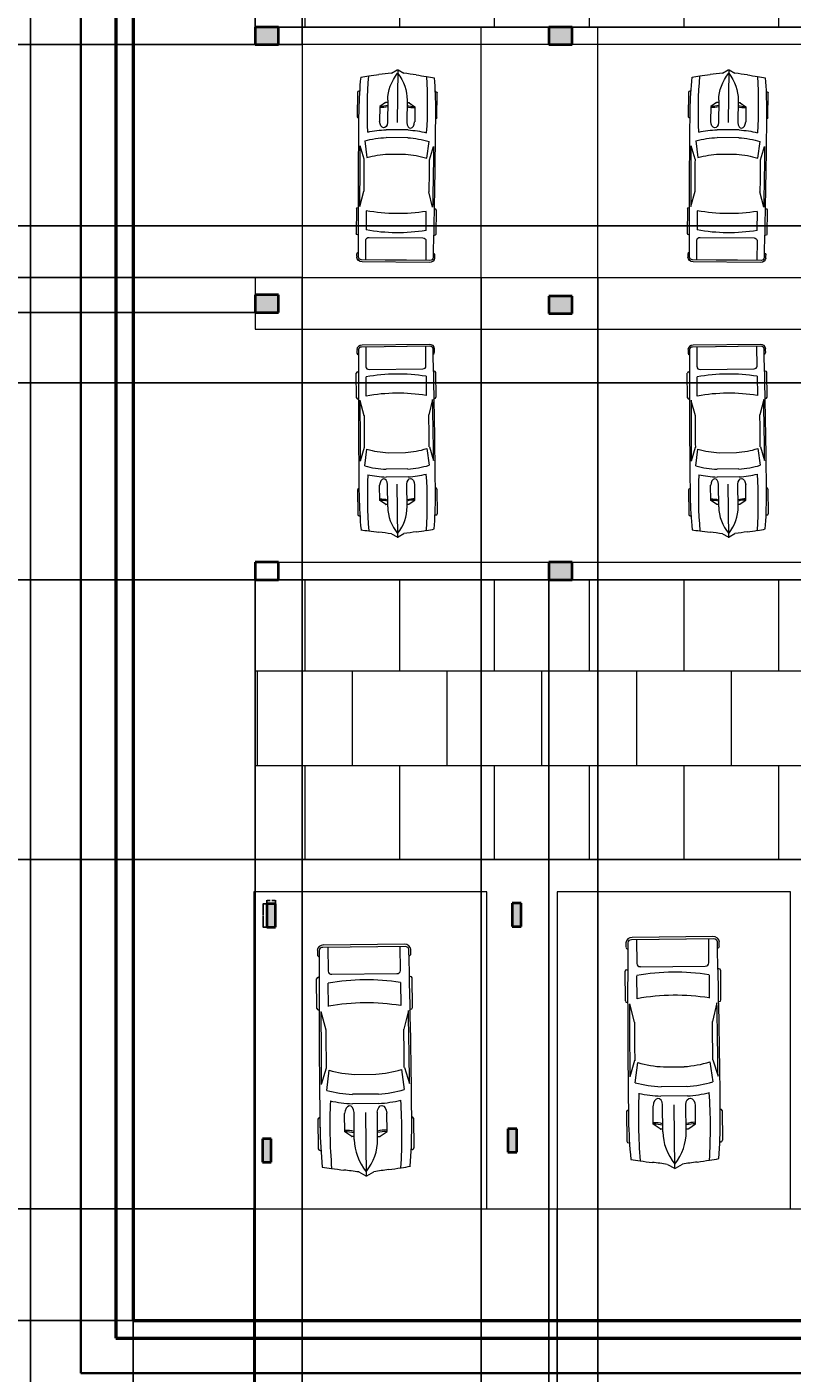
# Model space of a CAD drawing. Units: inches. Extents: x 154617 to 156384, y 250671 to 252576.
# Tile 3 of 6: x 155207 to 155601, y 251035 to 251728. Entities that reach past the tile are written whole.
import ezdxf

# ---------------------------------------------------------------- set-up
doc = ezdxf.new("R2010")
doc.units = ezdxf.units.IN
for name, color, linetype, lineweight in [('A-ANNO-DIMS', 2, 'Continuous', 18), ('A-EQPM-VEHI', 9, 'Continuous', 13), ('A-FLOR-DRIV', 5, 'Continuous', 25), ('A-FLOR-PATT', 112, 'Continuous', 13), ('A-FLOR-PRKG', 4, 'Continuous', 18), ('C-PROP', 5, 'Continuous', 35), ('C-ROAD', 7, 'Continuous', 25), ('pillars', 6, 'Continuous', 40), ('walls', 4, 'Continuous', 50)]:
    doc.layers.add(name, color=color, linetype=linetype, lineweight=lineweight)
doc.styles.get("Standard").update_dxf_attribs({"font": 'arial.ttf'})
doc.dimstyles.get("Standard").update_dxf_attribs({"dimtxt": 0.18, "dimasz": 0.18, "dimexe": 0.18, "dimexo": 0.0625, "dimgap": 0.09, "dimtad": 0, "dimtih": 1, "dimtoh": 1, "dimdec": 4, "dimzin": 0, "dimdsep": 46, "dimtxsty": 'Standard', "dimcen": 0.09, "dimadec": 0, "dimazin": 0, "dimtfac": 1, "dimtdec": 4, "dimtofl": 0, "dimtmove": 0, "dimatfit": 3, "dimfxl": 1, "dimtolj": 1, "dimtzin": 0, "dimarcsym": 0})

# ---------------------------------------------------------------- blocks, each defined once
blk = doc.blocks.new('*U2')
for p, q in [((21.1, 37.4), (21.1, 36.8)), ((46.6, 38.9), (22.4, 38.9)), ((47.8, 37.4), (47.8, 37.4)), ((88, 31.9), (74.8, 35.9)), ((134.3, 35.6), (119.3, 31.8)), ((135.5, 37.1), (135.5, 37.4)), ((136.7, 38.9), (160.9, 38.9)), ((162.1, 37.4), (162.1, 36.8)), ((186.5, -33.5), (186.5, 33.5)), ((70, 31.5), (86.4, 29.4)), ((138.4, 29.4), (157.2, 29.4)), ((164.5, 26.4), (164.5, -26.4)), ((186.5, 29.4), (167, 29.4)), ((188.4, -32.8), (188.4, 32.8)), ((32.1, 9.5), (32.1, 11.2)), ((32.3, 11.6), (36.1, 17.2)), ((36.1, 17.2), (50.9, 17.2)), ((3.3, 6.1), (0.1, 0.4)), ((29.8, 9.5), (51.7, 9.5)), ((58.9, -10.8), (58.9, 10.8)), ((66.6, -10.5), (66.6, 10.5)), ((82.7, 8.5), (82.7, -8.5)), ((186.5, -10.5), (186.5, 10.5)), ((0, 0), (51.7, 0)), ((0.1, -0.4), (3.3, -6.1)), ((29.8, -9.5), (51.7, -9.5)), ((32.1, -9.5), (32.1, -11.2)), ((32.3, -11.6), (36.1, -17.2)), ((36.1, -17.2), (50.9, -17.2)), ((86.4, -29.4), (70, -31.5)), ((88, -31.9), (74.8, -35.9)), ((134.3, -35.6), (119.3, -31.8)), ((157.2, -29.4), (138.4, -29.4)), ((167, -29.4), (186.5, -29.4)), ((21.1, -37.4), (21.1, -36.8)), ((46.6, -38.9), (22.4, -38.9)), ((47.8, -37.4), (47.8, -37.4)), ((135.5, -37.1), (135.5, -37.4)), ((136.7, -38.9), (160.9, -38.9)), ((162.1, -37.4), (162.1, -36.8))]:
    blk.add_line(p, q)
for centre, major_axis, ratio, start_param, end_param in [((266, -27.5), (0, 313.3), 0.842304, 1.367076, 1.39176), ((41.2, -490.9), (0, 528.2), 0.842304, 0.00281, 0.075598), ((22.4, 37.4), (0, -1.48), 0.842304, 3.141593, 4.712389), ((64.5, -10555.6), (0, 10593), 0.842304, -0.013397, 0.002797), ((46.6, 37.4), (0, 1.48), 0.842304, -1.570796, 0), ((64.5, -10555.6), (0, -10591.5), 0.842304, 3.133765, 3.140441), ((136.7, 37.4), (0, -1.48), 0.842304, 3.141593, 4.712389), ((160.9, 37.4), (0, 1.48), 0.842304, -1.570796, 0), ((180.6, 35.8), (0, 2.22), 0.842304, -0.013017, 1.249894), ((64.5, -10556.4), (0, 10595.3), 0.842304, -0.013397, -0.013017), ((184, 32.8), (0, -5.25), 0.842304, 1.570796, 3.128196), ((184, 33.5), (0, -2.96), 0.842304, 1.570796, 3.128196), ((259.2, -27.5), (0, -305.3), 0.842304, 4.528606, 4.561838), ((37.5, -594), (0, -623.3), 0.842304, 3.096046, 3.200911), ((134.4, 5.4), (0, -89.8), 0.842304, 4.449482, 4.652344), ((135.3, 5.4), (0, 81.8), 0.842304, 1.245306, 1.50788), ((149.6, 2.8), (0, -79.6), 0.842304, 4.372215, 4.640744), ((95.8, -3666.4), (0, -3698.2), 0.842304, 3.134049, 3.144098), ((17.1, 0), (0, 147), 0.842304, 4.511394, 4.913384), ((35.9, 0), (0, 147), 0.842304, 4.511394, 4.913384), ((167, 26.4), (0, 2.96), 0.842304, 0, 1.570796), ((-204.5, 52.4), (0, -251), 0.842304, 1.385369, 1.434372), ((32.7, 11.2), (0, 0.74), 0.842304, 0.879714, 1.570796), ((13, 17), (0, 27.4), 0.842304, 4.435146, 4.718221), ((14.2, 17), (0, 27.4), 0.842304, 4.435146, 4.718221), ((50.8, 13.3), (6.34, -0.36), 0.603834, -1.395552, 1.581315), ((0.6, 0), (0, -0.74), 0.842304, 4.131459, 5.293319), ((29.8, -46.7), (0, 56.2), 0.842304, 0, 0.590319), ((-204.5, -52.4), (0, 251), 0.842304, -1.434372, -1.385369), ((29.8, 46.7), (0, 56.2), 0.842304, 2.551274, 3.141593), ((13, -17), (0, -27.4), 0.842304, 1.564964, 1.848039), ((14.2, -17), (0, -27.4), 0.842304, 1.564964, 1.848039), ((134.4, -5.4), (0, -89.8), 0.842304, -1.510751, -1.307889), ((135.3, -5.4), (0, -81.8), 0.842304, -1.50788, -1.245306), ((149.6, -2.8), (0, -79.6), 0.842304, -1.499151, -1.230623), ((259.2, 27.5), (0, 305.3), 0.842304, 1.721348, 1.754579), ((32.7, -11.2), (0, -0.74), 0.842304, 4.712389, 5.403472), ((266, 27.5), (0, 313.3), 0.842304, 1.749832, 1.774517), ((37.5, 594), (0, -623.3), 0.842304, -0.059319, 0.045547), ((95.8, 3666.4), (0, -3698.2), 0.842304, -0.002505, 0.007544), ((167, -26.4), (0, -2.96), 0.842304, 4.712389, 6.283185), ((184, -32.8), (0, -5.25), 0.842304, 0.013397, 1.570796), ((41.2, 490.9), (0, -528.2), 0.842304, -0.075598, -0.00281), ((22.4, -37.4), (0, 1.48), 0.842304, 1.570796, 3.141593), ((64.5, 10555.6), (0, 10593), 0.842304, 3.138796, 3.15499), ((46.6, -37.4), (0, -1.48), 0.842304, 0, 1.570796), ((64.5, 10555.6), (0, -10591.5), 0.842304, 0.001152, 0.007828), ((136.7, -37.4), (0, -1.48), 0.842304, -1.570796, 0), ((160.9, -37.4), (0, 1.48), 0.842304, 3.141593, 4.712389), ((180.6, -35.8), (0, -2.22), 0.842304, -1.249894, 0.013017), ((64.5, 10556.4), (0, 10595.3), 0.842304, 3.15461, 3.15499), ((184, -33.5), (0, 2.96), 0.842304, 3.15499, 4.712389)]:
    blk.add_ellipse(centre, major_axis=major_axis, ratio=ratio, start_param=start_param, end_param=end_param)
at = {"extrusion": (0, 0, -1)}
blk.add_ellipse((50.8, -13.3), major_axis=(6.34, 0.36), ratio=0.603834, start_param=-1.395552, end_param=1.581315, dxfattribs=at)
blk = doc.blocks.new('COL-RECT-12x9')
h = blk.add_hatch(color=256)
h.dxf.hatch_style = 1
h.paths.add_polyline_path([(12.01, 0), (12.01, 9), (0, 9), (0, 0)])
for p, q in [((12.01, 9), (0, 9)), ((0, 9), (0, 0)), ((12.01, 0), (12.01, 9)), ((0, 0), (12.01, 0))]:
    blk.add_line(p, q)
blk = doc.blocks.new('COL-NARROW-4_5x12')
h = blk.add_hatch(color=256)
h.dxf.hatch_style = 1
h.paths.add_polyline_path([(4.5, 12.01), (0, 12.01), (0, 0), (4.5, 0)])
for p, q in [((4.5, 12.01), (0, 12.01)), ((0, 12.01), (0, 0)), ((4.5, 0), (4.5, 12.01)), ((0, 0), (4.5, 0))]:
    blk.add_line(p, q)
blk = doc.blocks.new('PARKING-BAY-U')
for p, q in [((120, 163.22), (0, 163.22)), ((0, 163.22), (0, 0)), ((120, 0), (120, 163.22))]:
    blk.add_line(p, q)
blk = doc.blocks.new('*D13')
at = {"layer": 'A-ANNO-DIMS', "color": 0, "lineweight": -2, "transparency": 16777216}
for p, q in [((155330.71, 251276.59), (155328.79, 251276.59)), ((155328.97, 251276.41), (155328.97, 251270.76)), ((155330.71, 251264.57), (155328.79, 251264.57)), ((155328.97, 251264.75), (155328.97, 251270.4))]:
    blk.add_line(p, q, dxfattribs=at)
at = {"layer": 'A-ANNO-DIMS', "color": 0, "transparency": 16777216}
for points in [[(155328.94, 251276.41), (155329, 251276.41), (155328.97, 251276.59)], [(155328.94, 251264.75), (155329, 251264.75), (155328.97, 251264.57)]]:
    blk.add_solid(points, dxfattribs=at)
at = {"layer": 'Defpoints', "color": 0, "transparency": 16777216}
for p in [(155330.77, 251276.59), (155328.97, 251264.57), (155330.77, 251264.57)]:
    blk.add_point(p, dxfattribs=at)
at = {"layer": 'A-ANNO-DIMS', "color": 0, "transparency": 16777216, "insert": (155328.97, 251270.58), "char_height": 0.18, "attachment_point": 5}
blk.add_mtext('\\A1;COLUMN 12 TYP.', dxfattribs=at)
blk = doc.blocks.new('*D14')
at = {"layer": 'A-ANNO-DIMS', "color": 0, "lineweight": -2, "transparency": 16777216}
for p, q in [((155330.77, 251276.65), (155330.77, 251278.57)), ((155330.95, 251278.39), (155332.56, 251278.39)), ((155335.09, 251278.39), (155333.48, 251278.39)), ((155335.27, 251276.65), (155335.27, 251278.57))]:
    blk.add_line(p, q, dxfattribs=at)
at = {"layer": 'A-ANNO-DIMS', "color": 0, "transparency": 16777216}
for points in [[(155330.95, 251278.42), (155330.95, 251278.36), (155330.77, 251278.39)], [(155335.09, 251278.42), (155335.09, 251278.36), (155335.27, 251278.39)]]:
    blk.add_solid(points, dxfattribs=at)
at = {"layer": 'Defpoints', "color": 0, "transparency": 16777216}
for p in [(155330.77, 251278.39), (155330.77, 251276.59), (155335.27, 251276.59)]:
    blk.add_point(p, dxfattribs=at)
at = {"layer": 'A-ANNO-DIMS', "color": 0, "transparency": 16777216, "insert": (155333.02, 251278.39), "char_height": 0.18, "attachment_point": 5}
blk.add_mtext('\\A1;5 TYP.', dxfattribs=at)
blk = doc.blocks.new('*D30')
at = {"layer": 'A-ANNO-DIMS', "color": 0, "lineweight": -2, "transparency": 16777216}
for p, q in [((155324.78, 251581.16), (154616.73, 251581.16)), ((154616.91, 251580.98), (154616.91, 251512.53)), ((154616.91, 251443.71), (154616.91, 251512.16)), ((155324.78, 251443.53), (154616.73, 251443.53))]:
    blk.add_line(p, q, dxfattribs=at)
at = {"layer": 'A-ANNO-DIMS', "color": 0, "transparency": 16777216}
for points in [[(154616.88, 251580.98), (154616.94, 251580.98), (154616.91, 251581.16)], [(154616.88, 251443.71), (154616.94, 251443.71), (154616.91, 251443.53)]]:
    blk.add_solid(points, dxfattribs=at)
at = {"layer": 'Defpoints', "color": 0, "transparency": 16777216}
for p in [(154616.91, 251581.16), (155324.84, 251581.16), (155324.84, 251443.53)]:
    blk.add_point(p, dxfattribs=at)
at = {"layer": 'A-ANNO-DIMS', "color": 0, "transparency": 16777216, "insert": (154616.91, 251512.35), "char_height": 0.18, "attachment_point": 5}
blk.add_mtext('\\A1;137.64', dxfattribs=at)
blk = doc.blocks.new('*D31')
at = {"layer": 'A-ANNO-DIMS', "color": 0, "lineweight": -2, "transparency": 16777216}
for p, q in [((155324.78, 251719.03), (154616.73, 251719.03)), ((154616.91, 251718.85), (154616.91, 251650.28)), ((154616.91, 251581.34), (154616.91, 251649.91)), ((155324.78, 251581.16), (154616.73, 251581.16))]:
    blk.add_line(p, q, dxfattribs=at)
at = {"layer": 'A-ANNO-DIMS', "color": 0, "transparency": 16777216}
for points in [[(154616.88, 251718.85), (154616.94, 251718.85), (154616.91, 251719.03)], [(154616.88, 251581.34), (154616.94, 251581.34), (154616.91, 251581.16)]]:
    blk.add_solid(points, dxfattribs=at)
at = {"layer": 'Defpoints', "color": 0, "transparency": 16777216}
for p in [(154616.91, 251719.03), (155324.84, 251719.03), (155324.84, 251581.16)]:
    blk.add_point(p, dxfattribs=at)
at = {"layer": 'A-ANNO-DIMS', "color": 0, "transparency": 16777216, "insert": (154616.91, 251650.1), "char_height": 0.18, "attachment_point": 5}
blk.add_mtext('\\A1;137.86', dxfattribs=at)
blk = doc.blocks.new('*D32')
at = {"layer": 'A-ANNO-DIMS', "color": 0, "lineweight": -2, "transparency": 16777216}
for p, q in [((155324.78, 251873.03), (154616.73, 251873.03)), ((154616.91, 251872.85), (154616.91, 251796.21)), ((154616.91, 251719.21), (154616.91, 251795.84)), ((155324.78, 251719.03), (154616.73, 251719.03))]:
    blk.add_line(p, q, dxfattribs=at)
at = {"layer": 'A-ANNO-DIMS', "color": 0, "transparency": 16777216}
for points in [[(154616.88, 251872.85), (154616.94, 251872.85), (154616.91, 251873.03)], [(154616.88, 251719.21), (154616.94, 251719.21), (154616.91, 251719.03)]]:
    blk.add_solid(points, dxfattribs=at)
at = {"layer": 'Defpoints', "color": 0, "transparency": 16777216}
for p in [(154616.91, 251873.03), (155324.84, 251873.03), (155324.84, 251719.03)]:
    blk.add_point(p, dxfattribs=at)
at = {"layer": 'A-ANNO-DIMS', "color": 0, "transparency": 16777216, "insert": (154616.91, 251796.03), "char_height": 0.18, "attachment_point": 5}
blk.add_mtext('\\A1;154', dxfattribs=at)
blk = doc.blocks.new('*D33')
at = {"layer": 'A-ANNO-DIMS', "color": 0, "lineweight": -2, "transparency": 16777216}
for p, q in [((155324.78, 251443.53), (154616.73, 251443.53)), ((154616.91, 251443.35), (154616.91, 251371.71)), ((154616.91, 251299.71), (154616.91, 251371.35)), ((155324.78, 251299.53), (154616.73, 251299.53))]:
    blk.add_line(p, q, dxfattribs=at)
at = {"layer": 'A-ANNO-DIMS', "color": 0, "transparency": 16777216}
for points in [[(154616.88, 251443.35), (154616.94, 251443.35), (154616.91, 251443.53)], [(154616.88, 251299.71), (154616.94, 251299.71), (154616.91, 251299.53)]]:
    blk.add_solid(points, dxfattribs=at)
at = {"layer": 'Defpoints', "color": 0, "transparency": 16777216}
for p in [(154616.91, 251443.53), (155324.84, 251443.53), (155324.84, 251299.53)]:
    blk.add_point(p, dxfattribs=at)
at = {"layer": 'A-ANNO-DIMS', "color": 0, "transparency": 16777216, "insert": (154616.91, 251371.53), "char_height": 0.18, "attachment_point": 5}
blk.add_mtext('\\A1;144', dxfattribs=at)
blk = doc.blocks.new('*D34')
at = {"layer": 'A-ANNO-DIMS', "color": 0, "lineweight": -2, "transparency": 16777216}
for p, q in [((155324.78, 251299.53), (154616.73, 251299.53)), ((154616.91, 251299.35), (154616.91, 251209.71)), ((154616.91, 251119.71), (154616.91, 251209.34)), ((155324, 251119.53), (154616.73, 251119.53))]:
    blk.add_line(p, q, dxfattribs=at)
at = {"layer": 'A-ANNO-DIMS', "color": 0, "transparency": 16777216}
for points in [[(154616.88, 251299.35), (154616.94, 251299.35), (154616.91, 251299.53)], [(154616.88, 251119.71), (154616.94, 251119.71), (154616.91, 251119.53)]]:
    blk.add_solid(points, dxfattribs=at)
at = {"layer": 'Defpoints', "color": 0, "transparency": 16777216}
for p in [(154616.91, 251299.53), (155324.84, 251299.53), (155324.06, 251119.53)]:
    blk.add_point(p, dxfattribs=at)
at = {"layer": 'A-ANNO-DIMS', "color": 0, "transparency": 16777216, "insert": (154616.91, 251209.53), "char_height": 0.18, "attachment_point": 5}
blk.add_mtext('\\A1;180', dxfattribs=at)
blk = doc.blocks.new('*D35')
at = {"layer": 'A-ANNO-DIMS', "color": 0, "lineweight": -2, "transparency": 16777216}
for p, q in [((155262.03, 251119.53), (154616.73, 251119.53)), ((154616.91, 251119.35), (154616.91, 251090.96)), ((154616.91, 251062.21), (154616.91, 251090.59)), ((155262.03, 251062.03), (154616.73, 251062.03))]:
    blk.add_line(p, q, dxfattribs=at)
at = {"layer": 'A-ANNO-DIMS', "color": 0, "transparency": 16777216}
for points in [[(154616.88, 251119.35), (154616.94, 251119.35), (154616.91, 251119.53)], [(154616.88, 251062.21), (154616.94, 251062.21), (154616.91, 251062.03)]]:
    blk.add_solid(points, dxfattribs=at)
at = {"layer": 'Defpoints', "color": 0, "transparency": 16777216}
for p in [(154616.91, 251119.53), (155262.1, 251119.53), (155262.1, 251062.03)]:
    blk.add_point(p, dxfattribs=at)
at = {"layer": 'A-ANNO-DIMS', "color": 0, "transparency": 16777216, "insert": (154616.91, 251090.78), "char_height": 0.18, "attachment_point": 5}
blk.add_mtext('\\A1;57.5', dxfattribs=at)
blk = doc.blocks.new('*D36')
at = {"layer": 'A-ANNO-DIMS', "color": 0, "lineweight": -2, "transparency": 16777216}
for p, q in [((155324.84, 251443.46), (155324.84, 250671.2)), ((155475.98, 251443.46), (155475.98, 250671.2)), ((155325.02, 250671.38), (155399.96, 250671.38)), ((155475.8, 250671.38), (155400.87, 250671.38))]:
    blk.add_line(p, q, dxfattribs=at)
at = {"layer": 'A-ANNO-DIMS', "color": 0, "transparency": 16777216}
for points in [[(155325.02, 250671.41), (155325.02, 250671.35), (155324.84, 250671.38)], [(155475.8, 250671.41), (155475.8, 250671.35), (155475.98, 250671.38)]]:
    blk.add_solid(points, dxfattribs=at)
at = {"layer": 'Defpoints', "color": 0, "transparency": 16777216}
for p in [(155324.84, 251443.53), (155475.98, 251443.53), (155475.98, 250671.38)]:
    blk.add_point(p, dxfattribs=at)
at = {"layer": 'A-ANNO-DIMS', "color": 0, "transparency": 16777216, "insert": (155400.41, 250671.38), "char_height": 0.18, "attachment_point": 5}
blk.add_mtext('\\A1;151.14', dxfattribs=at)
blk = doc.blocks.new('*D37')
at = {"layer": 'A-ANNO-DIMS', "color": 0, "lineweight": -2, "transparency": 16777216}
for p, q in [((155475.98, 251443.46), (155475.98, 250671.2)), ((155654.61, 251443.46), (155654.61, 250671.2)), ((155476.16, 250671.38), (155564.84, 250671.38)), ((155654.43, 250671.38), (155565.75, 250671.38))]:
    blk.add_line(p, q, dxfattribs=at)
at = {"layer": 'A-ANNO-DIMS', "color": 0, "transparency": 16777216}
for points in [[(155476.16, 250671.41), (155476.16, 250671.35), (155475.98, 250671.38)], [(155654.43, 250671.41), (155654.43, 250671.35), (155654.61, 250671.38)]]:
    blk.add_solid(points, dxfattribs=at)
at = {"layer": 'Defpoints', "color": 0, "transparency": 16777216}
for p in [(155475.98, 251443.53), (155654.61, 251443.53), (155654.61, 250671.38)]:
    blk.add_point(p, dxfattribs=at)
at = {"layer": 'A-ANNO-DIMS', "color": 0, "transparency": 16777216, "insert": (155565.3, 250671.38), "char_height": 0.18, "attachment_point": 5}
blk.add_mtext('\\A1;178.63', dxfattribs=at)
blk = doc.blocks.new('*D40')
at = {"layer": 'A-ANNO-DIMS', "color": 0, "lineweight": -2, "transparency": 16777216}
for p, q in [((155262.1, 251119.46), (155262.1, 250671.2)), ((155324.06, 251119.46), (155324.06, 250671.2)), ((155262.28, 250671.38), (155292.69, 250671.38)), ((155323.88, 250671.38), (155293.47, 250671.38))]:
    blk.add_line(p, q, dxfattribs=at)
at = {"layer": 'A-ANNO-DIMS', "color": 0, "transparency": 16777216}
for points in [[(155262.28, 250671.41), (155262.28, 250671.35), (155262.1, 250671.38)], [(155323.88, 250671.41), (155323.88, 250671.35), (155324.06, 250671.38)]]:
    blk.add_solid(points, dxfattribs=at)
at = {"layer": 'Defpoints', "color": 0, "transparency": 16777216}
for p in [(155262.1, 251119.53), (155324.06, 251119.53), (155324.06, 250671.38)]:
    blk.add_point(p, dxfattribs=at)
at = {"layer": 'A-ANNO-DIMS', "color": 0, "transparency": 16777216, "insert": (155293.08, 250671.38), "char_height": 0.18, "attachment_point": 5}
blk.add_mtext('\\A1;61.97', dxfattribs=at)
blk = doc.blocks.new('*D55')
at = {"layer": 'A-ANNO-DIMS', "color": 0, "lineweight": -2, "transparency": 16777216}
for p, q in [((155844.53, 251625.8), (154616.73, 251625.8)), ((154616.91, 251625.62), (154616.91, 251585.48)), ((154616.91, 251544.98), (154616.91, 251585.12)), ((155844.53, 251544.8), (154616.73, 251544.8))]:
    blk.add_line(p, q, dxfattribs=at)
at = {"layer": 'A-ANNO-DIMS', "color": 0, "transparency": 16777216}
for points in [[(154616.88, 251625.62), (154616.94, 251625.62), (154616.91, 251625.8)], [(154616.88, 251544.98), (154616.94, 251544.98), (154616.91, 251544.8)]]:
    blk.add_solid(points, dxfattribs=at)
at = {"layer": 'Defpoints', "color": 0, "transparency": 16777216}
for p in [(154616.91, 251625.8), (155844.6, 251625.8), (155844.6, 251544.8)]:
    blk.add_point(p, dxfattribs=at)
at = {"layer": 'A-ANNO-DIMS', "color": 0, "transparency": 16777216, "insert": (154616.91, 251585.3), "char_height": 0.18, "attachment_point": 5}
blk.add_mtext('\\A1;81', dxfattribs=at)
blk = doc.blocks.new('*D56')
at = {"layer": 'A-ANNO-DIMS', "color": 0, "lineweight": -2, "transparency": 16777216}
for p, q in [((155324.06, 251119.46), (155324.06, 250671.2)), ((155480.24, 251119.46), (155480.24, 250671.2)), ((155324.24, 250671.38), (155401.7, 250671.38)), ((155480.06, 250671.38), (155402.61, 250671.38))]:
    blk.add_line(p, q, dxfattribs=at)
at = {"layer": 'A-ANNO-DIMS', "color": 0, "transparency": 16777216}
for points in [[(155324.24, 250671.41), (155324.24, 250671.35), (155324.06, 250671.38)], [(155480.06, 250671.41), (155480.06, 250671.35), (155480.24, 250671.38)]]:
    blk.add_solid(points, dxfattribs=at)
at = {"layer": 'Defpoints', "color": 0, "transparency": 16777216}
for p in [(155324.06, 251119.53), (155480.24, 251119.53), (155480.24, 250671.38)]:
    blk.add_point(p, dxfattribs=at)
at = {"layer": 'A-ANNO-DIMS', "color": 0, "transparency": 16777216, "insert": (155402.15, 250671.38), "char_height": 0.18, "attachment_point": 5}
blk.add_mtext('\\A1;156.18', dxfattribs=at)
blk = doc.blocks.new('*D57')
at = {"layer": 'A-ANNO-DIMS', "color": 0, "lineweight": -2, "transparency": 16777216}
for p, q in [((155480.24, 251119.46), (155480.24, 250671.2)), ((155608.93, 251119.46), (155608.93, 250671.2)), ((155480.42, 250671.38), (155544.13, 250671.38)), ((155608.75, 250671.38), (155545.04, 250671.38))]:
    blk.add_line(p, q, dxfattribs=at)
at = {"layer": 'A-ANNO-DIMS', "color": 0, "transparency": 16777216}
for points in [[(155480.42, 250671.41), (155480.42, 250671.35), (155480.24, 250671.38)], [(155608.75, 250671.41), (155608.75, 250671.35), (155608.93, 250671.38)]]:
    blk.add_solid(points, dxfattribs=at)
at = {"layer": 'Defpoints', "color": 0, "transparency": 16777216}
for p in [(155480.24, 251119.53), (155608.93, 251119.53), (155608.93, 250671.38)]:
    blk.add_point(p, dxfattribs=at)
at = {"layer": 'A-ANNO-DIMS', "color": 0, "transparency": 16777216, "insert": (155544.58, 250671.38), "char_height": 0.18, "attachment_point": 5}
blk.add_mtext('\\A1;128.68', dxfattribs=at)
blk = doc.blocks.new('*D59')
at = {"layer": 'A-ANNO-DIMS', "color": 0, "lineweight": -2, "transparency": 16777216}
for p, q in [((155348.98, 251598.96), (155348.98, 250671.2)), ((155441.1, 251598.96), (155441.1, 250671.2)), ((155349.16, 250671.38), (155394.65, 250671.38)), ((155440.92, 250671.38), (155395.43, 250671.38))]:
    blk.add_line(p, q, dxfattribs=at)
at = {"layer": 'A-ANNO-DIMS', "color": 0, "transparency": 16777216}
for points in [[(155349.16, 250671.41), (155349.16, 250671.35), (155348.98, 250671.38)], [(155440.92, 250671.41), (155440.92, 250671.35), (155441.1, 250671.38)]]:
    blk.add_solid(points, dxfattribs=at)
at = {"layer": 'Defpoints', "color": 0, "transparency": 16777216}
for p in [(155348.98, 251599.03), (155441.1, 251599.03), (155441.1, 250671.38)]:
    blk.add_point(p, dxfattribs=at)
at = {"layer": 'A-ANNO-DIMS', "color": 0, "transparency": 16777216, "insert": (155395.04, 250671.38), "char_height": 0.18, "attachment_point": 5}
blk.add_mtext('\\A1;92.12', dxfattribs=at)
blk = doc.blocks.new('*D60')
at = {"layer": 'A-ANNO-DIMS', "color": 0, "lineweight": -2, "transparency": 16777216}
for p, q in [((155441.1, 251598.96), (155441.1, 250671.2)), ((155501.1, 251598.96), (155501.1, 250671.2)), ((155441.28, 250671.38), (155470.88, 250671.38)), ((155500.92, 250671.38), (155471.32, 250671.38))]:
    blk.add_line(p, q, dxfattribs=at)
at = {"layer": 'A-ANNO-DIMS', "color": 0, "transparency": 16777216}
for points in [[(155441.28, 250671.41), (155441.28, 250671.35), (155441.1, 250671.38)], [(155500.92, 250671.41), (155500.92, 250671.35), (155501.1, 250671.38)]]:
    blk.add_solid(points, dxfattribs=at)
at = {"layer": 'Defpoints', "color": 0, "transparency": 16777216}
for p in [(155441.1, 251599.03), (155501.1, 251599.03), (155501.1, 250671.38)]:
    blk.add_point(p, dxfattribs=at)
at = {"layer": 'A-ANNO-DIMS', "color": 0, "transparency": 16777216, "insert": (155471.1, 250671.38), "char_height": 0.18, "attachment_point": 5}
blk.add_mtext('\\A1;60', dxfattribs=at)
blk = doc.blocks.new('*D61')
at = {"layer": 'A-ANNO-DIMS', "color": 0, "lineweight": -2, "transparency": 16777216}
for p, q in [((155501.1, 251598.96), (155501.1, 250671.2)), ((155621.1, 251598.96), (155621.1, 250671.2)), ((155501.28, 250671.38), (155560.82, 250671.38)), ((155620.92, 250671.38), (155561.38, 250671.38))]:
    blk.add_line(p, q, dxfattribs=at)
at = {"layer": 'A-ANNO-DIMS', "color": 0, "transparency": 16777216}
for points in [[(155501.28, 250671.41), (155501.28, 250671.35), (155501.1, 250671.38)], [(155620.92, 250671.41), (155620.92, 250671.35), (155621.1, 250671.38)]]:
    blk.add_solid(points, dxfattribs=at)
at = {"layer": 'Defpoints', "color": 0, "transparency": 16777216}
for p in [(155501.1, 251599.03), (155621.1, 251599.03), (155621.1, 250671.38)]:
    blk.add_point(p, dxfattribs=at)
at = {"layer": 'A-ANNO-DIMS', "color": 0, "transparency": 16777216, "insert": (155561.1, 250671.38), "char_height": 0.18, "attachment_point": 5}
blk.add_mtext('\\A1;120', dxfattribs=at)
blk = doc.blocks.new('*D62')
at = {"layer": 'A-ANNO-DIMS', "color": 0, "lineweight": -2, "transparency": 16777216}
for p, q in [((155348.92, 251719.03), (154616.73, 251719.03)), ((154616.91, 251718.85), (154616.91, 251659.21)), ((154616.91, 251599.21), (154616.91, 251658.84)), ((155348.92, 251599.03), (154616.73, 251599.03))]:
    blk.add_line(p, q, dxfattribs=at)
at = {"layer": 'A-ANNO-DIMS', "color": 0, "transparency": 16777216}
for points in [[(154616.88, 251718.85), (154616.94, 251718.85), (154616.91, 251719.03)], [(154616.88, 251599.21), (154616.94, 251599.21), (154616.91, 251599.03)]]:
    blk.add_solid(points, dxfattribs=at)
at = {"layer": 'Defpoints', "color": 0, "transparency": 16777216}
for p in [(154616.91, 251719.03), (155348.98, 251719.03), (155348.98, 251599.03)]:
    blk.add_point(p, dxfattribs=at)
at = {"layer": 'A-ANNO-DIMS', "color": 0, "transparency": 16777216, "insert": (154616.91, 251659.03), "char_height": 0.18, "attachment_point": 5}
blk.add_mtext('\\A1;120', dxfattribs=at)
blk = doc.blocks.new('*D67')
at = {"layer": 'A-ANNO-DIMS', "color": 0, "lineweight": -2, "transparency": 16777216}
for p, q in [((155324.84, 251719.09), (155324.84, 252576.18)), ((155325.02, 252576), (155336.52, 252576)), ((155348.8, 252576), (155337.31, 252576)), ((155348.98, 251719.09), (155348.98, 252576.18))]:
    blk.add_line(p, q, dxfattribs=at)
at = {"layer": 'A-ANNO-DIMS', "color": 0, "transparency": 16777216}
for points in [[(155325.02, 252576.03), (155325.02, 252575.97), (155324.84, 252576)], [(155348.8, 252576.03), (155348.8, 252575.97), (155348.98, 252576)]]:
    blk.add_solid(points, dxfattribs=at)
at = {"layer": 'Defpoints', "color": 0, "transparency": 16777216}
for p in [(155348.98, 252576), (155324.84, 251719.03), (155348.98, 251719.03)]:
    blk.add_point(p, dxfattribs=at)
at = {"layer": 'A-ANNO-DIMS', "color": 0, "transparency": 16777216, "insert": (155336.91, 252576), "char_height": 0.18, "attachment_point": 5}
blk.add_mtext('\\A1;24.14', dxfattribs=at)

msp = doc.modelspace()

# ---------------------------------------------------------------- hatches: boundary and pattern name
at = {"layer": 'A-FLOR-PATT'}
h = msp.add_hatch(dxfattribs=at)
h.set_pattern_fill('AR-B88', color=256, scale=0.24)
h.set_pattern_definition([(0, (0, -2.5), (0, 48.768), []), (90, (0, -2.5), (-24.384, 48.768), [48.768, -48.768])])
h.paths.add_polyline_path([(155324.842, 251443.526), (155324.842, 251299.526), (155945.097, 251299.526), (155945.097, 251119.526), (156089.097, 251119.526), (156089.097, 252132.026), (155921.097, 252132.026), (155921.097, 251872.026), (155324.842, 251872.026), (155324.842, 251728.026), (155921.097, 251728.026), (155921.097, 251443.526)])

# ---------------------------------------------------------------- linework, layer by layer
at = {"layer": 'A-FLOR-DRIV'}
for p, q in [((155921.097, 251728.026), (155324.842, 251728.026)), ((155324.842, 251728.026), (155324.842, 251719.026)), ((155324.842, 251452.526), (155324.842, 251299.526)), ((155324.842, 251443.526), (155921.097, 251443.526)), ((155324.842, 251299.526), (155945.097, 251299.526))]:
    msp.add_line(p, q, dxfattribs=at)
at = {"layer": 'A-FLOR-PRKG'}
for p, q in [((155441.097, 251599.026), (155441.097, 251728.026)), ((155501.097, 251599.026), (155501.097, 251728.026)), ((155921.097, 251719.026), (155324.842, 251719.026)), ((155348.982, 251719.026), (155348.982, 251599.026)), ((155741.097, 251599.026), (155324.842, 251599.026)), ((155324.842, 251599.026), (155324.842, 251572.526)), ((155324.842, 251572.526), (155741.097, 251572.526)), ((155348.982, 251572.526), (155348.982, 251452.526)), ((155441.097, 251443.526), (155441.097, 251572.526)), ((155501.097, 251443.526), (155501.097, 251572.526)), ((155324.842, 251452.526), (155921.097, 251452.526)), ((155262.097, 251119.526), (156089.097, 251119.526))]:
    msp.add_line(p, q, dxfattribs=at)
at = {"layer": 'C-PROP'}
for p, q in [((155235.097, 252221.526), (155235.097, 251035.026)), ((155235.097, 251035.026), (156296.097, 251035.026))]:
    msp.add_line(p, q, dxfattribs=at)
at = {"layer": 'C-ROAD'}
msp.add_line((155209.237, 252414.495), (155209.237, 250798.266), dxfattribs=at)
at = {"layer": 'pillars'}
for p, q in [((155336.855, 251452.526), (155324.842, 251452.526)), ((155324.842, 251452.526), (155324.842, 251443.526)), ((155336.855, 251443.526), (155336.855, 251452.526)), ((155324.842, 251443.526), (155336.855, 251443.526))]:
    msp.add_line(p, q, dxfattribs=at)
at = {"layer": 'walls'}
for p, q in [((155253.097, 252203.526), (155253.097, 251053.026)), ((155262.097, 252194.526), (155262.097, 251062.026)), ((155262.097, 251062.026), (156269.097, 251062.026)), ((155253.097, 251053.026), (156278.097, 251053.026))]:
    msp.add_line(p, q, dxfattribs=at)

# ---------------------------------------------------------------- block references
at = {"layer": 'A-EQPM-VEHI'}
for p, xscale, yscale, zscale, rotation in [((155398.165, 251706.094), -0.5257159977764584, 0.5257159977764584, 0.5257159977764584, 89.41840527650862), ((155568.511, 251706.094), -0.5257159977764584, 0.5257159977764584, 0.5257159977764584, 89.41840527650862), ((155398.165, 251465.459), 0.5257159977764584, 0.5257159977764584, 0.5257159977764584, 90.58159472349136), ((155568.511, 251465.459), 0.5257159977764584, 0.5257159977764584, 0.5257159977764584, 90.58159472349136), ((155540.8, 251140.453), 0.632208294406123, 0.632208294406123, 0.632208294406123, 90.58159472349136), ((155382.038, 251136.54), 0.632208294406123, 0.632208294406123, 0.632208294406123, 90.58159472349136)]:
    msp.add_blockref('*U2', p, dxfattribs=dict(at, xscale=xscale, yscale=yscale, zscale=zscale, rotation=rotation))
at = {"layer": 'A-FLOR-PRKG'}
for p in [(155324.064, 251119.526), (155480.245, 251119.526)]:
    msp.add_blockref('PARKING-BAY-U', p, dxfattribs=at)
at = {"layer": 'pillars'}
for p in [(155324.841, 251719.027), (155475.979, 251719.027), (155324.841, 251581.164), (155475.979, 251580.536), (155475.979, 251443.527)]:
    msp.add_blockref('COL-RECT-12x9', p, dxfattribs=at)
at = {"layer": 'pillars', "rotation": 180}
for p in [(155335.268, 251276.586), (155461.644, 251276.964), (155459.394, 251160.733), (155333.018, 251155.58)]:
    msp.add_blockref('COL-NARROW-4_5x12', p, dxfattribs=at)

# ---------------------------------------------------------------- dimensions: what is measured, and where the dimension line sits
at = {"layer": 'A-ANNO-DIMS'}
for base, p1, p2, override, picture, middle in [((155348.982, 252575.997), (155324.842, 251719.026), (155348.982, 251719.026), {"dimdec": 2, "dimlfac": 1, "dimrnd": 0, "dimzin": 0, "dimdsep": 46, "dimlunit": 2}, '*D67', (155336.912, 252575.997)), ((155441.0971, 250671.3791), (155348.9817, 251599.0264), (155441.0971, 251599.0264), {"dimdec": 2, "dimlfac": 1, "dimrnd": 0, "dimzin": 0, "dimdsep": 46, "dimlunit": 2}, '*D59', (155395.0394, 250671.3791)), ((155501.097, 250671.379), (155441.097, 251599.026), (155501.097, 251599.026), {"dimdec": 0, "dimlfac": 1, "dimrnd": 0, "dimzin": 0, "dimdsep": 46, "dimlunit": 2}, '*D60', (155471.097, 250671.379)), ((155621.097, 250671.379), (155501.097, 251599.026), (155621.097, 251599.026), {"dimdec": 0, "dimlfac": 1, "dimrnd": 0, "dimzin": 0, "dimdsep": 46, "dimlunit": 2}, '*D61', (155561.097, 250671.379)), ((155475.98, 250671.379), (155324.842, 251443.526), (155475.98, 251443.526), {"dimdec": 2, "dimlfac": 1, "dimrnd": 0, "dimzin": 0, "dimdsep": 46, "dimlunit": 2}, '*D36', (155400.411, 250671.379)), ((155654.613, 250671.379), (155475.98, 251443.526), (155654.613, 251443.526), {"dimdec": 2, "dimlfac": 1, "dimrnd": 0, "dimzin": 0, "dimdsep": 46, "dimlunit": 2}, '*D37', (155565.297, 250671.379)), ((155324.063, 250671.379), (155262.097, 251119.526), (155324.063, 251119.526), {"dimdec": 2, "dimlfac": 1, "dimrnd": 0, "dimzin": 0, "dimdsep": 46, "dimlunit": 2}, '*D40', (155293.08, 250671.379)), ((155480.244, 250671.379), (155324.063, 251119.526), (155480.244, 251119.526), {"dimdec": 2, "dimlfac": 1, "dimrnd": 0, "dimzin": 0, "dimdsep": 46, "dimlunit": 2}, '*D56', (155402.154, 250671.379)), ((155608.926, 250671.379), (155480.244, 251119.526), (155608.926, 251119.526), {"dimdec": 2, "dimlfac": 1, "dimrnd": 0, "dimzin": 0, "dimdsep": 46, "dimlunit": 2}, '*D57', (155544.585, 250671.379))]:
    dim = msp.add_linear_dim(base=base, p1=p1, p2=p2, dimstyle='Standard', override=override, dxfattribs=at)
    dim.commit()
    dim.dimension.update_dxf_attribs({"geometry": picture, "text_midpoint": middle})
for base, p1, p2, override, picture, middle in [((154616.915, 251873.026), (155324.842, 251719.026), (155324.842, 251873.026), {"dimdec": 0, "dimlfac": 1, "dimrnd": 0, "dimzin": 0, "dimdsep": 46, "dimlunit": 2}, '*D32', (154616.915, 251796.026)), ((154616.915, 251719.026), (155324.842, 251581.164), (155324.842, 251719.026), {"dimdec": 2, "dimlfac": 1, "dimrnd": 0, "dimzin": 0, "dimdsep": 46, "dimlunit": 2}, '*D31', (154616.915, 251650.095)), ((154616.915, 251719.026), (155348.982, 251599.026), (155348.982, 251719.026), {"dimdec": 0, "dimlfac": 1, "dimrnd": 0, "dimzin": 0, "dimdsep": 46, "dimlunit": 2}, '*D62', (154616.915, 251659.026)), ((154616.915, 251625.802), (155844.597, 251544.802), (155844.597, 251625.802), {"dimdec": 0, "dimlfac": 1, "dimrnd": 0, "dimzin": 0, "dimdsep": 46, "dimlunit": 2}, '*D55', (154616.915, 251585.302)), ((154616.915, 251581.164), (155324.842, 251443.526), (155324.842, 251581.164), {"dimdec": 2, "dimlfac": 1, "dimrnd": 0, "dimzin": 0, "dimdsep": 46, "dimlunit": 2}, '*D30', (154616.915, 251512.345)), ((154616.915, 251443.526), (155324.842, 251299.526), (155324.842, 251443.526), {"dimdec": 0, "dimlfac": 1, "dimrnd": 0, "dimzin": 0, "dimdsep": 46, "dimlunit": 2}, '*D33', (154616.915, 251371.526)), ((154616.915, 251299.526), (155324.063, 251119.526), (155324.842, 251299.526), {"dimdec": 0, "dimlfac": 1, "dimrnd": 0, "dimzin": 0, "dimdsep": 46, "dimlunit": 2}, '*D34', (154616.915, 251209.526)), ((154616.915, 251119.526), (155262.097, 251062.026), (155262.097, 251119.526), {"dimdec": 1, "dimlfac": 1, "dimrnd": 0, "dimzin": 0, "dimdsep": 46, "dimlunit": 2}, '*D35', (154616.915, 251090.776))]:
    dim = msp.add_linear_dim(base=base, p1=p1, p2=p2, angle=90, dimstyle='Standard', override=override, dxfattribs=at)
    dim.commit()
    dim.dimension.update_dxf_attribs({"geometry": picture, "text_midpoint": middle})
for base, p1, p2, angle, text, picture, middle in [((155330.768533694, 251278.387727271), (155335.268533694, 251276.585829146), (155330.768533694, 251276.585829146), 180, '<> TYP.', '*D14', (155333.018533694, 251278.387727271)), ((155328.967, 251264.573), (155330.769, 251276.586), (155330.769, 251264.573), 270, 'COLUMN <> TYP.', '*D13', (155328.967, 251270.58))]:
    dim = msp.add_linear_dim(base=base, p1=p1, p2=p2, angle=angle, text=text, dimstyle='Standard', override={"dimdec": 0, "dimlfac": 1, "dimrnd": 0, "dimzin": 0, "dimdsep": 46, "dimlunit": 2}, dxfattribs=at)
    dim.commit()
    dim.dimension.update_dxf_attribs({"geometry": picture, "text_midpoint": middle})

doc.saveas('drawing.dxf')
